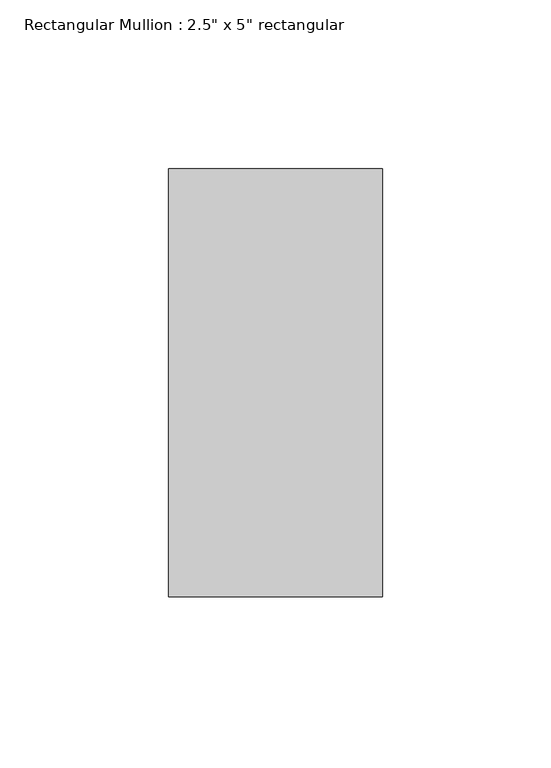
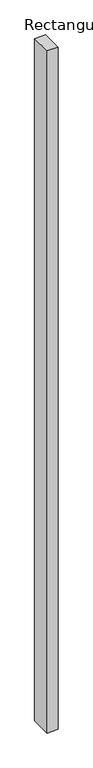
"""IFC4 building model written with IfcOpenShell, lengths in millimetres: member geometry."""

from ifc_helpers import new_model, si_unit, frame, origin, place, context, project, spatial, polyline, outline, extrude, source, transform, mapped, element, save


def member_623a4a38(model_context):
    return source(origin(), model_context, "Body", "SweptSolid", [
        extrude(outline(polyline([(0.0, 63.5), (0.0, -63.5), (-63.5, -63.5), (-63.5, 63.5), (0.0, 63.5)])), frame((0.0, 0.0, -4216.4), z_axis=(0.0, 0.0, 1.0), x_axis=(1.0, 0.0, 0.0)), (0.0, 0.0, 1.0), 4216.4),
    ])


if __name__ == "__main__":
    model = new_model("IFC4")
    model_context = context("Model", 3, world=origin())
    ifc_project = project(units=[si_unit("LENGTHUNIT", "METRE", prefix="MILLI")], contexts=[model_context])
    site = spatial("IfcSite", under=ifc_project)
    building = spatial("IfcBuilding", under=site)
    placement = place(None, origin())
    member_shape = member_623a4a38(model_context)
    element("IfcMember", 1, ObjectType="Rectangular Mullion : 2.5\" x 5\" rectangular", at=placement, inside=building, context=model_context, shape_type="MappedRepresentation", body=[
        mapped(member_shape, transform((0.0, 0.0, 0.0), x_axis=(1.0, 0.0, 0.0), y_axis=(0.0, 1.0, 0.0), z_axis=(0.0, 0.0, 1.0))),
    ])
    save(model, "model.ifc")

# Revit data of these elements
# Type "Rectangular Mullion : 2.5\" x 5\" rectangular"
#   built-in parameter 1007304 = 0.416667 (stored number, unit not read)
#   built-in parameter 1007301 = 0.104167 (stored number, unit not read)
#   built-in parameter 1007300 = 0.104167 (stored number, unit not read)
# Element 1 (IfcMember, "Rectangular Mullion : 2.5\" x 5\" rectangular")
#   Materials on its faces: "Aluminum"
# Materials
#   "Aluminum": class "Metal", colour RGB 247 247 247, transparency 0, Description = "Aluminum 6061", Cost = 0
